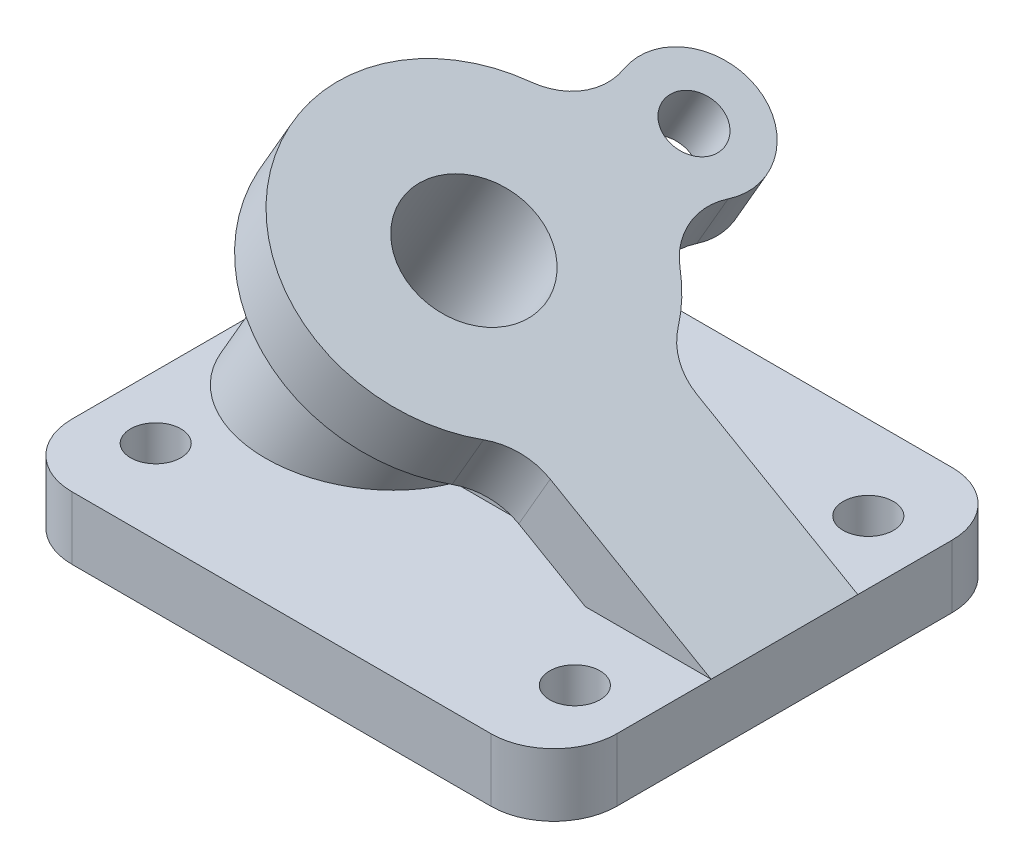
ISO-10303-21;
HEADER;
FILE_DESCRIPTION(('STEP AP214'),'2;1');
FILE_NAME('part.step','',(''),(''),'','','');
FILE_SCHEMA(('AUTOMOTIVE_DESIGN { 1 0 10303 214 1 1 1 1 }'));
ENDSEC;
DATA;
#1=APPLICATION_CONTEXT('core data for automotive mechanical design processes');
#2=APPLICATION_PROTOCOL_DEFINITION('international standard','automotive_design',2000,#1);
#3=PRODUCT_CONTEXT('',#1,'mechanical');
#4=PRODUCT('Part','Part','',(#3));
#5=PRODUCT_RELATED_PRODUCT_CATEGORY('part','',(#4));
#6=PRODUCT_DEFINITION_FORMATION('','',#4);
#7=PRODUCT_DEFINITION_CONTEXT('part definition',#1,'design');
#8=PRODUCT_DEFINITION('design','',#6,#7);
#9=PRODUCT_DEFINITION_SHAPE('','',#8);
#10=(LENGTH_UNIT() NAMED_UNIT(*) SI_UNIT(.MILLI.,.METRE.));
#11=(NAMED_UNIT(*) PLANE_ANGLE_UNIT() SI_UNIT($,.RADIAN.));
#12=(NAMED_UNIT(*) SI_UNIT($,.STERADIAN.) SOLID_ANGLE_UNIT());
#13=UNCERTAINTY_MEASURE_WITH_UNIT(LENGTH_MEASURE(1.E-05),#10,'distance_accuracy_value','');
#14=(GEOMETRIC_REPRESENTATION_CONTEXT(3) GLOBAL_UNCERTAINTY_ASSIGNED_CONTEXT((#13)) GLOBAL_UNIT_ASSIGNED_CONTEXT((#10,
#11,#12)) REPRESENTATION_CONTEXT('',''));
#15=CARTESIAN_POINT('',(0.,0.,0.));
#16=DIRECTION('',(0.,0.,1.));
#17=DIRECTION('',(1.,0.,0.));
#18=AXIS2_PLACEMENT_3D('',#15,#16,#17);
#19=CARTESIAN_POINT('',(50.,15.,40.));
#20=DIRECTION('',(0.,1.,0.));
#21=DIRECTION('',(0.,0.,1.));
#22=AXIS2_PLACEMENT_3D('',#19,#20,#21);
#23=PLANE('',#22);
#24=DIRECTION('',(1.,0.,0.));
#25=VECTOR('',#24,1.);
#26=CARTESIAN_POINT('',(50.,15.,17.5));
#27=LINE('',#26,#25);
#28=CARTESIAN_POINT('',(34.9999999999997,15.,17.5));
#29=VERTEX_POINT('',#28);
#30=CARTESIAN_POINT('',(65.,15.,17.5));
#31=VERTEX_POINT('',#30);
#32=EDGE_CURVE('E56',#29,#31,#27,.T.);
#33=ORIENTED_EDGE('',*,*,#32,.F.);
#34=DIRECTION('',(0.,0.,-1.));
#35=VECTOR('',#34,1.);
#36=CARTESIAN_POINT('',(34.9999999999997,15.,40.));
#37=LINE('',#36,#35);
#38=CARTESIAN_POINT('',(34.9999999999996,15.,7.5));
#39=VERTEX_POINT('',#38);
#40=EDGE_CURVE('E213',#29,#39,#37,.T.);
#41=ORIENTED_EDGE('',*,*,#40,.T.);
#42=DIRECTION('',(-1.,0.,0.));
#43=VECTOR('',#42,1.);
#44=CARTESIAN_POINT('',(-16.2509999999997,15.,7.5));
#45=LINE('',#44,#43);
#46=CARTESIAN_POINT('',(-6.24198056079765,15.,7.5));
#47=VERTEX_POINT('',#46);
#48=EDGE_CURVE('E304',#39,#47,#45,.T.);
#49=ORIENTED_EDGE('',*,*,#48,.T.);
#50=CARTESIAN_POINT('',(-33.7798332972281,15.,0.));
#51=DIRECTION('',(0.,1.,0.));
#52=DIRECTION('',(1.,0.,0.));
#53=AXIS2_PLACEMENT_3D('',#50,#51,#52);
#54=ELLIPSE('',#53,28.8675134594812,25.);
#55=CARTESIAN_POINT('',(-6.24198056079765,15.,-7.5));
#56=VERTEX_POINT('',#55);
#57=EDGE_CURVE('E300',#56,#47,#54,.T.);
#58=ORIENTED_EDGE('',*,*,#57,.F.);
#59=DIRECTION('',(-1.,0.,0.));
#60=VECTOR('',#59,1.);
#61=CARTESIAN_POINT('',(-16.2509999999997,15.,-7.5));
#62=LINE('',#61,#60);
#63=CARTESIAN_POINT('',(34.9999999999996,15.,-7.5));
#64=VERTEX_POINT('',#63);
#65=EDGE_CURVE('E298',#64,#56,#62,.T.);
#66=ORIENTED_EDGE('',*,*,#65,.F.);
#67=CARTESIAN_POINT('',(34.9999999999997,15.,-17.5));
#68=VERTEX_POINT('',#67);
#69=EDGE_CURVE('E68',#64,#68,#37,.T.);
#70=ORIENTED_EDGE('',*,*,#69,.T.);
#71=DIRECTION('',(1.,0.,0.));
#72=VECTOR('',#71,1.);
#73=CARTESIAN_POINT('',(50.,15.,-17.5));
#74=LINE('',#73,#72);
#75=CARTESIAN_POINT('',(65.,15.,-17.5));
#76=VERTEX_POINT('',#75);
#77=EDGE_CURVE('E284',#68,#76,#74,.T.);
#78=ORIENTED_EDGE('',*,*,#77,.T.);
#79=DIRECTION('',(0.,0.,-1.));
#80=VECTOR('',#79,1.);
#81=CARTESIAN_POINT('',(65.,15.,-39.9999999999999));
#82=LINE('',#81,#80);
#83=CARTESIAN_POINT('',(65.,15.,-39.9999999999999));
#84=VERTEX_POINT('',#83);
#85=EDGE_CURVE('E335',#76,#84,#82,.T.);
#86=ORIENTED_EDGE('',*,*,#85,.T.);
#87=CARTESIAN_POINT('',(50.,15.,-40.));
#88=DIRECTION('',(0.,1.,0.));
#89=DIRECTION('',(0.,0.,-1.));
#90=AXIS2_PLACEMENT_3D('',#87,#88,#89);
#91=CIRCLE('',#90,15.);
#92=CARTESIAN_POINT('',(49.9999999999999,15.,-55.));
#93=VERTEX_POINT('',#92);
#94=EDGE_CURVE('E338',#84,#93,#91,.T.);
#95=ORIENTED_EDGE('',*,*,#94,.T.);
#96=DIRECTION('',(-1.,0.,0.));
#97=VECTOR('',#96,1.);
#98=CARTESIAN_POINT('',(-49.9999999999999,15.,-55.));
#99=LINE('',#98,#97);
#100=CARTESIAN_POINT('',(-49.9999999999999,15.,-55.));
#101=VERTEX_POINT('',#100);
#102=EDGE_CURVE('E337',#93,#101,#99,.T.);
#103=ORIENTED_EDGE('',*,*,#102,.T.);
#104=CARTESIAN_POINT('',(-50.,15.,-40.));
#105=DIRECTION('',(0.,1.,0.));
#106=DIRECTION('',(0.,0.,1.));
#107=AXIS2_PLACEMENT_3D('',#104,#105,#106);
#108=CIRCLE('',#107,15.);
#109=CARTESIAN_POINT('',(-65.,15.,-39.9999999999999));
#110=VERTEX_POINT('',#109);
#111=EDGE_CURVE('E336',#101,#110,#108,.T.);
#112=ORIENTED_EDGE('',*,*,#111,.T.);
#113=DIRECTION('',(0.,0.,1.));
#114=VECTOR('',#113,1.);
#115=CARTESIAN_POINT('',(-65.,15.,-39.9999999999999));
#116=LINE('',#115,#114);
#117=CARTESIAN_POINT('',(-65.,15.,39.9999999999999));
#118=VERTEX_POINT('',#117);
#119=EDGE_CURVE('E344',#110,#118,#116,.T.);
#120=ORIENTED_EDGE('',*,*,#119,.T.);
#121=CARTESIAN_POINT('',(-50.,15.,40.));
#122=DIRECTION('',(0.,1.,0.));
#123=DIRECTION('',(0.,0.,1.));
#124=AXIS2_PLACEMENT_3D('',#121,#122,#123);
#125=CIRCLE('',#124,15.);
#126=CARTESIAN_POINT('',(-49.9999999999999,15.,55.));
#127=VERTEX_POINT('',#126);
#128=EDGE_CURVE('E345',#118,#127,#125,.T.);
#129=ORIENTED_EDGE('',*,*,#128,.T.);
#130=DIRECTION('',(1.,0.,0.));
#131=VECTOR('',#130,1.);
#132=CARTESIAN_POINT('',(-49.9999999999999,15.,55.));
#133=LINE('',#132,#131);
#134=CARTESIAN_POINT('',(49.9999999999999,15.,55.));
#135=VERTEX_POINT('',#134);
#136=EDGE_CURVE('E347',#127,#135,#133,.T.);
#137=ORIENTED_EDGE('',*,*,#136,.T.);
#138=CARTESIAN_POINT('',(50.,15.,40.));
#139=DIRECTION('',(0.,1.,0.));
#140=DIRECTION('',(0.,0.,1.));
#141=AXIS2_PLACEMENT_3D('',#138,#139,#140);
#142=CIRCLE('',#141,15.);
#143=CARTESIAN_POINT('',(65.,15.,39.9999999999999));
#144=VERTEX_POINT('',#143);
#145=EDGE_CURVE('E328',#135,#144,#142,.T.);
#146=ORIENTED_EDGE('',*,*,#145,.T.);
#147=EDGE_CURVE('E331',#144,#31,#82,.T.);
#148=ORIENTED_EDGE('',*,*,#147,.T.);
#149=EDGE_LOOP('',(#33,#41,#49,#58,#66,#70,#78,#86,#95,#103,#112,#120,#129,#137,#146,#148));
#150=FACE_BOUND('',#149,.T.);
#151=CARTESIAN_POINT('',(50.,15.,35.));
#152=DIRECTION('',(0.,1.,0.));
#153=DIRECTION('',(0.,0.,-1.));
#154=AXIS2_PLACEMENT_3D('',#151,#152,#153);
#155=CIRCLE('',#154,6.);
#156=CARTESIAN_POINT('',(50.,15.,29.));
#157=VERTEX_POINT('',#156);
#158=EDGE_CURVE('E313',#157,#157,#155,.T.);
#159=ORIENTED_EDGE('',*,*,#158,.F.);
#160=EDGE_LOOP('',(#159));
#161=FACE_BOUND('',#160,.T.);
#162=CARTESIAN_POINT('',(-50.,15.,-35.));
#163=DIRECTION('',(0.,1.,0.));
#164=DIRECTION('',(0.,0.,1.));
#165=AXIS2_PLACEMENT_3D('',#162,#163,#164);
#166=CIRCLE('',#165,6.);
#167=CARTESIAN_POINT('',(-50.,15.,-29.));
#168=VERTEX_POINT('',#167);
#169=EDGE_CURVE('E323',#168,#168,#166,.T.);
#170=ORIENTED_EDGE('',*,*,#169,.F.);
#171=EDGE_LOOP('',(#170));
#172=FACE_BOUND('',#171,.T.);
#173=CARTESIAN_POINT('',(-50.,15.,35.));
#174=DIRECTION('',(0.,1.,0.));
#175=DIRECTION('',(0.,0.,1.));
#176=AXIS2_PLACEMENT_3D('',#173,#174,#175);
#177=CIRCLE('',#176,6.);
#178=CARTESIAN_POINT('',(-50.,15.,41.));
#179=VERTEX_POINT('',#178);
#180=EDGE_CURVE('E320',#179,#179,#177,.T.);
#181=ORIENTED_EDGE('',*,*,#180,.F.);
#182=EDGE_LOOP('',(#181));
#183=FACE_BOUND('',#182,.T.);
#184=CARTESIAN_POINT('',(50.,15.,-35.));
#185=DIRECTION('',(0.,1.,0.));
#186=DIRECTION('',(0.,0.,-1.));
#187=AXIS2_PLACEMENT_3D('',#184,#185,#186);
#188=CIRCLE('',#187,6.);
#189=CARTESIAN_POINT('',(50.,15.,-41.));
#190=VERTEX_POINT('',#189);
#191=EDGE_CURVE('E301',#190,#190,#188,.T.);
#192=ORIENTED_EDGE('',*,*,#191,.F.);
#193=EDGE_LOOP('',(#192));
#194=FACE_BOUND('',#193,.T.);
#195=ADVANCED_FACE('F43',(#150,#161,#172,#183,#194),#23,.T.);
#196=CARTESIAN_POINT('',(50.,0.,40.));
#197=DIRECTION('',(0.,1.,0.));
#198=DIRECTION('',(0.,0.,1.));
#199=AXIS2_PLACEMENT_3D('',#196,#197,#198);
#200=PLANE('',#199);
#201=CARTESIAN_POINT('',(50.,0.,40.));
#202=DIRECTION('',(0.,1.,0.));
#203=DIRECTION('',(0.,0.,1.));
#204=AXIS2_PLACEMENT_3D('',#201,#202,#203);
#205=CIRCLE('',#204,15.);
#206=CARTESIAN_POINT('',(49.9999999999999,0.,55.));
#207=VERTEX_POINT('',#206);
#208=CARTESIAN_POINT('',(65.,0.,39.9999999999999));
#209=VERTEX_POINT('',#208);
#210=EDGE_CURVE('E326',#207,#209,#205,.T.);
#211=ORIENTED_EDGE('',*,*,#210,.F.);
#212=DIRECTION('',(1.,0.,0.));
#213=VECTOR('',#212,1.);
#214=CARTESIAN_POINT('',(-49.9999999999999,0.,55.));
#215=LINE('',#214,#213);
#216=CARTESIAN_POINT('',(-49.9999999999999,0.,55.));
#217=VERTEX_POINT('',#216);
#218=EDGE_CURVE('E334',#217,#207,#215,.T.);
#219=ORIENTED_EDGE('',*,*,#218,.F.);
#220=CARTESIAN_POINT('',(-50.,0.,40.));
#221=DIRECTION('',(0.,1.,0.));
#222=DIRECTION('',(0.,0.,1.));
#223=AXIS2_PLACEMENT_3D('',#220,#221,#222);
#224=CIRCLE('',#223,15.);
#225=CARTESIAN_POINT('',(-65.,0.,39.9999999999999));
#226=VERTEX_POINT('',#225);
#227=EDGE_CURVE('E363',#226,#217,#224,.T.);
#228=ORIENTED_EDGE('',*,*,#227,.F.);
#229=DIRECTION('',(0.,0.,1.));
#230=VECTOR('',#229,1.);
#231=CARTESIAN_POINT('',(-65.,0.,-39.9999999999999));
#232=LINE('',#231,#230);
#233=CARTESIAN_POINT('',(-65.,0.,-39.9999999999999));
#234=VERTEX_POINT('',#233);
#235=EDGE_CURVE('E360',#234,#226,#232,.T.);
#236=ORIENTED_EDGE('',*,*,#235,.F.);
#237=CARTESIAN_POINT('',(-50.,0.,-40.));
#238=DIRECTION('',(0.,1.,0.));
#239=DIRECTION('',(0.,0.,1.));
#240=AXIS2_PLACEMENT_3D('',#237,#238,#239);
#241=CIRCLE('',#240,15.);
#242=CARTESIAN_POINT('',(-49.9999999999999,0.,-55.));
#243=VERTEX_POINT('',#242);
#244=EDGE_CURVE('E359',#243,#234,#241,.T.);
#245=ORIENTED_EDGE('',*,*,#244,.F.);
#246=DIRECTION('',(-1.,0.,0.));
#247=VECTOR('',#246,1.);
#248=CARTESIAN_POINT('',(-49.9999999999999,0.,-55.));
#249=LINE('',#248,#247);
#250=CARTESIAN_POINT('',(49.9999999999999,0.,-55.));
#251=VERTEX_POINT('',#250);
#252=EDGE_CURVE('E351',#251,#243,#249,.T.);
#253=ORIENTED_EDGE('',*,*,#252,.F.);
#254=CARTESIAN_POINT('',(50.,0.,-40.));
#255=DIRECTION('',(0.,1.,0.));
#256=DIRECTION('',(0.,0.,-1.));
#257=AXIS2_PLACEMENT_3D('',#254,#255,#256);
#258=CIRCLE('',#257,15.);
#259=CARTESIAN_POINT('',(65.,0.,-39.9999999999999));
#260=VERTEX_POINT('',#259);
#261=EDGE_CURVE('E352',#260,#251,#258,.T.);
#262=ORIENTED_EDGE('',*,*,#261,.F.);
#263=DIRECTION('',(0.,0.,-1.));
#264=VECTOR('',#263,1.);
#265=CARTESIAN_POINT('',(65.,0.,-39.9999999999999));
#266=LINE('',#265,#264);
#267=EDGE_CURVE('E353',#209,#260,#266,.T.);
#268=ORIENTED_EDGE('',*,*,#267,.F.);
#269=EDGE_LOOP('',(#211,#219,#228,#236,#245,#253,#262,#268));
#270=FACE_BOUND('',#269,.T.);
#271=CARTESIAN_POINT('',(-50.,0.,-35.));
#272=DIRECTION('',(0.,1.,0.));
#273=DIRECTION('',(0.,0.,1.));
#274=AXIS2_PLACEMENT_3D('',#271,#272,#273);
#275=CIRCLE('',#274,6.);
#276=CARTESIAN_POINT('',(-50.,0.,-29.));
#277=VERTEX_POINT('',#276);
#278=EDGE_CURVE('E319',#277,#277,#275,.T.);
#279=ORIENTED_EDGE('',*,*,#278,.T.);
#280=EDGE_LOOP('',(#279));
#281=FACE_BOUND('',#280,.T.);
#282=CARTESIAN_POINT('',(-50.,0.,35.));
#283=DIRECTION('',(0.,1.,0.));
#284=DIRECTION('',(0.,0.,1.));
#285=AXIS2_PLACEMENT_3D('',#282,#283,#284);
#286=CIRCLE('',#285,6.);
#287=CARTESIAN_POINT('',(-50.,0.,41.));
#288=VERTEX_POINT('',#287);
#289=EDGE_CURVE('E314',#288,#288,#286,.T.);
#290=ORIENTED_EDGE('',*,*,#289,.T.);
#291=EDGE_LOOP('',(#290));
#292=FACE_BOUND('',#291,.T.);
#293=CARTESIAN_POINT('',(50.,0.,35.));
#294=DIRECTION('',(0.,1.,0.));
#295=DIRECTION('',(0.,0.,-1.));
#296=AXIS2_PLACEMENT_3D('',#293,#294,#295);
#297=CIRCLE('',#296,6.);
#298=CARTESIAN_POINT('',(50.,0.,29.));
#299=VERTEX_POINT('',#298);
#300=EDGE_CURVE('E306',#299,#299,#297,.T.);
#301=ORIENTED_EDGE('',*,*,#300,.T.);
#302=EDGE_LOOP('',(#301));
#303=FACE_BOUND('',#302,.T.);
#304=CARTESIAN_POINT('',(50.,0.,-35.));
#305=DIRECTION('',(0.,1.,0.));
#306=DIRECTION('',(0.,0.,-1.));
#307=AXIS2_PLACEMENT_3D('',#304,#305,#306);
#308=CIRCLE('',#307,6.);
#309=CARTESIAN_POINT('',(50.,0.,-41.));
#310=VERTEX_POINT('',#309);
#311=EDGE_CURVE('E302',#310,#310,#308,.T.);
#312=ORIENTED_EDGE('',*,*,#311,.T.);
#313=EDGE_LOOP('',(#312));
#314=FACE_BOUND('',#313,.T.);
#315=ADVANCED_FACE('F398',(#270,#281,#292,#303,#314),#200,.F.);
#316=CARTESIAN_POINT('',(50.,15.,40.));
#317=DIRECTION('',(0.,-1.,0.));
#318=DIRECTION('',(0.,0.,-1.));
#319=AXIS2_PLACEMENT_3D('',#316,#317,#318);
#320=CYLINDRICAL_SURFACE('',#319,15.);
#321=ORIENTED_EDGE('',*,*,#210,.T.);
#322=DIRECTION('',(0.,-1.,0.));
#323=VECTOR('',#322,1.);
#324=CARTESIAN_POINT('',(65.,15.,39.9999999999999));
#325=LINE('',#324,#323);
#326=EDGE_CURVE('E50',#144,#209,#325,.T.);
#327=ORIENTED_EDGE('',*,*,#326,.F.);
#328=ORIENTED_EDGE('',*,*,#145,.F.);
#329=DIRECTION('',(0.,-1.,0.));
#330=VECTOR('',#329,1.);
#331=CARTESIAN_POINT('',(49.9999999999999,15.,55.));
#332=LINE('',#331,#330);
#333=EDGE_CURVE('E346',#135,#207,#332,.T.);
#334=ORIENTED_EDGE('',*,*,#333,.T.);
#335=EDGE_LOOP('',(#321,#327,#328,#334));
#336=FACE_BOUND('',#335,.T.);
#337=ADVANCED_FACE('F44',(#336),#320,.T.);
#338=CARTESIAN_POINT('',(65.,15.,-39.9999999999999));
#339=DIRECTION('',(-1.,0.,0.));
#340=DIRECTION('',(0.,0.,1.));
#341=AXIS2_PLACEMENT_3D('',#338,#339,#340);
#342=PLANE('',#341);
#343=ORIENTED_EDGE('',*,*,#267,.T.);
#344=DIRECTION('',(0.,-1.,0.));
#345=VECTOR('',#344,1.);
#346=CARTESIAN_POINT('',(65.,15.,-39.9999999999999));
#347=LINE('',#346,#345);
#348=EDGE_CURVE('E379',#84,#260,#347,.T.);
#349=ORIENTED_EDGE('',*,*,#348,.F.);
#350=ORIENTED_EDGE('',*,*,#85,.F.);
#351=DIRECTION('',(0.,0.,-1.));
#352=VECTOR('',#351,1.);
#353=CARTESIAN_POINT('',(65.,15.,0.));
#354=LINE('',#353,#352);
#355=EDGE_CURVE('E239',#31,#76,#354,.T.);
#356=ORIENTED_EDGE('',*,*,#355,.F.);
#357=ORIENTED_EDGE('',*,*,#147,.F.);
#358=ORIENTED_EDGE('',*,*,#326,.T.);
#359=EDGE_LOOP('',(#343,#349,#350,#356,#357,#358));
#360=FACE_BOUND('',#359,.T.);
#361=ADVANCED_FACE('F386',(#360),#342,.F.);
#362=CARTESIAN_POINT('',(50.,15.,-40.));
#363=DIRECTION('',(0.,-1.,0.));
#364=DIRECTION('',(0.,0.,-1.));
#365=AXIS2_PLACEMENT_3D('',#362,#363,#364);
#366=CYLINDRICAL_SURFACE('',#365,15.);
#367=ORIENTED_EDGE('',*,*,#261,.T.);
#368=DIRECTION('',(0.,-1.,0.));
#369=VECTOR('',#368,1.);
#370=CARTESIAN_POINT('',(49.9999999999999,15.,-55.));
#371=LINE('',#370,#369);
#372=EDGE_CURVE('E378',#93,#251,#371,.T.);
#373=ORIENTED_EDGE('',*,*,#372,.F.);
#374=ORIENTED_EDGE('',*,*,#94,.F.);
#375=ORIENTED_EDGE('',*,*,#348,.T.);
#376=EDGE_LOOP('',(#367,#373,#374,#375));
#377=FACE_BOUND('',#376,.T.);
#378=ADVANCED_FACE('F405',(#377),#366,.T.);
#379=CARTESIAN_POINT('',(-49.9999999999999,15.,-55.));
#380=DIRECTION('',(0.,0.,1.));
#381=DIRECTION('',(1.,0.,0.));
#382=AXIS2_PLACEMENT_3D('',#379,#380,#381);
#383=PLANE('',#382);
#384=ORIENTED_EDGE('',*,*,#252,.T.);
#385=DIRECTION('',(0.,-1.,0.));
#386=VECTOR('',#385,1.);
#387=CARTESIAN_POINT('',(-49.9999999999999,15.,-55.));
#388=LINE('',#387,#386);
#389=EDGE_CURVE('E374',#101,#243,#388,.T.);
#390=ORIENTED_EDGE('',*,*,#389,.F.);
#391=ORIENTED_EDGE('',*,*,#102,.F.);
#392=ORIENTED_EDGE('',*,*,#372,.T.);
#393=EDGE_LOOP('',(#384,#390,#391,#392));
#394=FACE_BOUND('',#393,.T.);
#395=ADVANCED_FACE('F403',(#394),#383,.F.);
#396=CARTESIAN_POINT('',(-50.,15.,-40.));
#397=DIRECTION('',(0.,-1.,0.));
#398=DIRECTION('',(0.,0.,-1.));
#399=AXIS2_PLACEMENT_3D('',#396,#397,#398);
#400=CYLINDRICAL_SURFACE('',#399,15.);
#401=ORIENTED_EDGE('',*,*,#244,.T.);
#402=DIRECTION('',(0.,-1.,0.));
#403=VECTOR('',#402,1.);
#404=CARTESIAN_POINT('',(-65.,15.,-39.9999999999999));
#405=LINE('',#404,#403);
#406=EDGE_CURVE('E375',#110,#234,#405,.T.);
#407=ORIENTED_EDGE('',*,*,#406,.F.);
#408=ORIENTED_EDGE('',*,*,#111,.F.);
#409=ORIENTED_EDGE('',*,*,#389,.T.);
#410=EDGE_LOOP('',(#401,#407,#408,#409));
#411=FACE_BOUND('',#410,.T.);
#412=ADVANCED_FACE('F666',(#411),#400,.T.);
#413=CARTESIAN_POINT('',(-65.,15.,-39.9999999999999));
#414=DIRECTION('',(1.,0.,0.));
#415=DIRECTION('',(0.,0.,-1.));
#416=AXIS2_PLACEMENT_3D('',#413,#414,#415);
#417=PLANE('',#416);
#418=ORIENTED_EDGE('',*,*,#235,.T.);
#419=DIRECTION('',(0.,-1.,0.));
#420=VECTOR('',#419,1.);
#421=CARTESIAN_POINT('',(-65.,15.,39.9999999999999));
#422=LINE('',#421,#420);
#423=EDGE_CURVE('E369',#118,#226,#422,.T.);
#424=ORIENTED_EDGE('',*,*,#423,.F.);
#425=ORIENTED_EDGE('',*,*,#119,.F.);
#426=ORIENTED_EDGE('',*,*,#406,.T.);
#427=EDGE_LOOP('',(#418,#424,#425,#426));
#428=FACE_BOUND('',#427,.T.);
#429=ADVANCED_FACE('F659',(#428),#417,.F.);
#430=CARTESIAN_POINT('',(-50.,15.,40.));
#431=DIRECTION('',(0.,-1.,0.));
#432=DIRECTION('',(0.,0.,-1.));
#433=AXIS2_PLACEMENT_3D('',#430,#431,#432);
#434=CYLINDRICAL_SURFACE('',#433,15.);
#435=ORIENTED_EDGE('',*,*,#227,.T.);
#436=DIRECTION('',(0.,-1.,0.));
#437=VECTOR('',#436,1.);
#438=CARTESIAN_POINT('',(-49.9999999999999,15.,55.));
#439=LINE('',#438,#437);
#440=EDGE_CURVE('E368',#127,#217,#439,.T.);
#441=ORIENTED_EDGE('',*,*,#440,.F.);
#442=ORIENTED_EDGE('',*,*,#128,.F.);
#443=ORIENTED_EDGE('',*,*,#423,.T.);
#444=EDGE_LOOP('',(#435,#441,#442,#443));
#445=FACE_BOUND('',#444,.T.);
#446=ADVANCED_FACE('F649',(#445),#434,.T.);
#447=CARTESIAN_POINT('',(-49.9999999999999,15.,55.));
#448=DIRECTION('',(0.,0.,-1.));
#449=DIRECTION('',(-1.,0.,0.));
#450=AXIS2_PLACEMENT_3D('',#447,#448,#449);
#451=PLANE('',#450);
#452=ORIENTED_EDGE('',*,*,#218,.T.);
#453=ORIENTED_EDGE('',*,*,#333,.F.);
#454=ORIENTED_EDGE('',*,*,#136,.F.);
#455=ORIENTED_EDGE('',*,*,#440,.T.);
#456=EDGE_LOOP('',(#452,#453,#454,#455));
#457=FACE_BOUND('',#456,.T.);
#458=ADVANCED_FACE('F643',(#457),#451,.F.);
#459=CARTESIAN_POINT('',(-50.,15.,-35.));
#460=DIRECTION('',(0.,-1.,0.));
#461=DIRECTION('',(0.,0.,-1.));
#462=AXIS2_PLACEMENT_3D('',#459,#460,#461);
#463=CYLINDRICAL_SURFACE('',#462,6.);
#464=ORIENTED_EDGE('',*,*,#169,.T.);
#465=EDGE_LOOP('',(#464));
#466=FACE_BOUND('',#465,.T.);
#467=ORIENTED_EDGE('',*,*,#278,.F.);
#468=EDGE_LOOP('',(#467));
#469=FACE_BOUND('',#468,.T.);
#470=ADVANCED_FACE('F633',(#466,#469),#463,.F.);
#471=CARTESIAN_POINT('',(-50.,15.,35.));
#472=DIRECTION('',(0.,-1.,0.));
#473=DIRECTION('',(0.,0.,-1.));
#474=AXIS2_PLACEMENT_3D('',#471,#472,#473);
#475=CYLINDRICAL_SURFACE('',#474,6.);
#476=ORIENTED_EDGE('',*,*,#180,.T.);
#477=EDGE_LOOP('',(#476));
#478=FACE_BOUND('',#477,.T.);
#479=ORIENTED_EDGE('',*,*,#289,.F.);
#480=EDGE_LOOP('',(#479));
#481=FACE_BOUND('',#480,.T.);
#482=ADVANCED_FACE('F622',(#478,#481),#475,.F.);
#483=CARTESIAN_POINT('',(50.,15.,35.));
#484=DIRECTION('',(0.,-1.,0.));
#485=DIRECTION('',(0.,0.,-1.));
#486=AXIS2_PLACEMENT_3D('',#483,#484,#485);
#487=CYLINDRICAL_SURFACE('',#486,6.);
#488=ORIENTED_EDGE('',*,*,#158,.T.);
#489=EDGE_LOOP('',(#488));
#490=FACE_BOUND('',#489,.T.);
#491=ORIENTED_EDGE('',*,*,#300,.F.);
#492=EDGE_LOOP('',(#491));
#493=FACE_BOUND('',#492,.T.);
#494=ADVANCED_FACE('F461',(#490,#493),#487,.F.);
#495=CARTESIAN_POINT('',(50.,15.,-35.));
#496=DIRECTION('',(0.,-1.,0.));
#497=DIRECTION('',(0.,0.,-1.));
#498=AXIS2_PLACEMENT_3D('',#495,#496,#497);
#499=CYLINDRICAL_SURFACE('',#498,6.);
#500=ORIENTED_EDGE('',*,*,#191,.T.);
#501=EDGE_LOOP('',(#500));
#502=FACE_BOUND('',#501,.T.);
#503=ORIENTED_EDGE('',*,*,#311,.F.);
#504=EDGE_LOOP('',(#503));
#505=FACE_BOUND('',#504,.T.);
#506=ADVANCED_FACE('F451',(#502,#505),#499,.F.);
#507=CARTESIAN_POINT('',(-48.0810655013041,-9.77046078830035,0.));
#508=DIRECTION('',(0.499999999999995,0.866025403784442,0.));
#509=DIRECTION('',(-0.866025403784442,0.499999999999995,0.));
#510=AXIS2_PLACEMENT_3D('',#507,#508,#509);
#511=CYLINDRICAL_SURFACE('',#510,25.);
#512=DIRECTION('',(0.499999999999995,0.866025403784442,0.));
#513=VECTOR('',#512,1.);
#514=CARTESIAN_POINT('',(-27.4276759489812,-21.694700806012,-7.50000000000001));
#515=LINE('',#514,#513);
#516=CARTESIAN_POINT('',(4.06851457940145,32.8583014340171,-7.5));
#517=VERTEX_POINT('',#516);
#518=EDGE_CURVE('E295',#56,#517,#515,.T.);
#519=ORIENTED_EDGE('',*,*,#518,.F.);
#520=ORIENTED_EDGE('',*,*,#57,.T.);
#521=DIRECTION('',(0.499999999999995,0.866025403784442,0.));
#522=VECTOR('',#521,1.);
#523=CARTESIAN_POINT('',(-27.4276759489812,-21.694700806012,7.49999999999999));
#524=LINE('',#523,#522);
#525=CARTESIAN_POINT('',(4.06851457940146,32.8583014340171,7.5));
#526=VERTEX_POINT('',#525);
#527=EDGE_CURVE('E294',#47,#526,#524,.T.);
#528=ORIENTED_EDGE('',*,*,#527,.T.);
#529=CARTESIAN_POINT('',(-16.5848749729215,44.7825414517288,0.));
#530=DIRECTION('',(-0.499999999999995,-0.866025403784442,0.));
#531=DIRECTION('',(0.866025403784442,-0.499999999999995,0.));
#532=AXIS2_PLACEMENT_3D('',#529,#530,#531);
#533=CIRCLE('',#532,25.);
#534=EDGE_CURVE('E288',#526,#517,#533,.T.);
#535=ORIENTED_EDGE('',*,*,#534,.T.);
#536=EDGE_LOOP('',(#519,#520,#528,#535));
#537=FACE_BOUND('',#536,.T.);
#538=ADVANCED_FACE('F447',(#537),#511,.T.);
#539=CARTESIAN_POINT('',(-16.2509999999997,-28.1475576738016,-7.50000000000001));
#540=DIRECTION('',(0.,0.,1.));
#541=DIRECTION('',(0.,-1.,0.));
#542=AXIS2_PLACEMENT_3D('',#539,#540,#541);
#543=PLANE('',#542);
#544=DIRECTION('',(0.866025403784442,-0.499999999999995,0.));
#545=VECTOR('',#544,1.);
#546=CARTESIAN_POINT('',(15.245190528383,26.4054445662275,-7.5));
#547=LINE('',#546,#545);
#548=EDGE_CURVE('E290',#517,#64,#547,.T.);
#549=ORIENTED_EDGE('',*,*,#548,.T.);
#550=ORIENTED_EDGE('',*,*,#65,.T.);
#551=ORIENTED_EDGE('',*,*,#518,.T.);
#552=EDGE_LOOP('',(#549,#550,#551));
#553=FACE_BOUND('',#552,.T.);
#554=ADVANCED_FACE('F443',(#553),#543,.F.);
#555=CARTESIAN_POINT('',(-16.2509999999997,-28.1475576738016,7.49999999999999));
#556=DIRECTION('',(0.,0.,1.));
#557=DIRECTION('',(0.,-1.,0.));
#558=AXIS2_PLACEMENT_3D('',#555,#556,#557);
#559=PLANE('',#558);
#560=ORIENTED_EDGE('',*,*,#48,.F.);
#561=DIRECTION('',(0.866025403784442,-0.499999999999995,0.));
#562=VECTOR('',#561,1.);
#563=CARTESIAN_POINT('',(15.245190528383,26.4054445662275,7.5));
#564=LINE('',#563,#562);
#565=EDGE_CURVE('E285',#526,#39,#564,.T.);
#566=ORIENTED_EDGE('',*,*,#565,.F.);
#567=ORIENTED_EDGE('',*,*,#527,.F.);
#568=EDGE_LOOP('',(#560,#566,#567));
#569=FACE_BOUND('',#568,.T.);
#570=ADVANCED_FACE('F454',(#569),#559,.T.);
#571=CARTESIAN_POINT('',(15.245190528383,26.4054445662275,0.));
#572=DIRECTION('',(0.499999999999995,0.866025403784442,0.));
#573=DIRECTION('',(-0.866025403784442,0.499999999999995,0.));
#574=AXIS2_PLACEMENT_3D('',#571,#572,#573);
#575=PLANE('',#574);
#576=ORIENTED_EDGE('',*,*,#69,.F.);
#577=ORIENTED_EDGE('',*,*,#548,.F.);
#578=ORIENTED_EDGE('',*,*,#534,.F.);
#579=ORIENTED_EDGE('',*,*,#565,.T.);
#580=ORIENTED_EDGE('',*,*,#40,.F.);
#581=DIRECTION('',(0.866025403784442,-0.499999999999995,0.));
#582=VECTOR('',#581,1.);
#583=CARTESIAN_POINT('',(15.245190528383,26.4054445662275,17.5));
#584=LINE('',#583,#582);
#585=CARTESIAN_POINT('',(19.1222671697929,24.1670133236407,17.5));
#586=VERTEX_POINT('',#585);
#587=EDGE_CURVE('E194',#586,#29,#584,.T.);
#588=ORIENTED_EDGE('',*,*,#587,.F.);
#589=CARTESIAN_POINT('',(19.1222671697929,24.1670133236407,32.5));
#590=DIRECTION('',(0.499999999999995,0.866025403784442,0.));
#591=DIRECTION('',(-0.866025403784442,0.499999999999995,0.));
#592=AXIS2_PLACEMENT_3D('',#589,#590,#591);
#593=CIRCLE('',#592,15.);
#594=CARTESIAN_POINT('',(8.92022655758879,30.0571642173801,23.2142857142857));
#595=VERTEX_POINT('',#594);
#596=EDGE_CURVE('E205',#586,#595,#593,.T.);
#597=ORIENTED_EDGE('',*,*,#596,.T.);
#598=CARTESIAN_POINT('',(-16.5848749729215,44.7825414517288,0.));
#599=DIRECTION('',(0.499999999999995,0.866025403784442,0.));
#600=DIRECTION('',(-0.866025403784442,0.499999999999995,0.));
#601=AXIS2_PLACEMENT_3D('',#598,#599,#600);
#602=CIRCLE('',#601,37.5);
#603=CARTESIAN_POINT('',(-34.3689821748944,55.0502005320849,-31.3775510204082));
#604=VERTEX_POINT('',#603);
#605=EDGE_CURVE('E234',#604,#595,#602,.T.);
#606=ORIENTED_EDGE('',*,*,#605,.F.);
#607=CARTESIAN_POINT('',(-41.4826250556835,59.1572641642273,-43.9285714285714));
#608=DIRECTION('',(0.499999999999995,0.866025403784442,0.));
#609=DIRECTION('',(-0.866025403784442,0.499999999999995,0.));
#610=AXIS2_PLACEMENT_3D('',#607,#608,#609);
#611=CIRCLE('',#610,15.);
#612=CARTESIAN_POINT('',(-29.0337500143025,51.969902807978,-48.2142857142857));
#613=VERTEX_POINT('',#612);
#614=EDGE_CURVE('E226',#604,#613,#611,.T.);
#615=ORIENTED_EDGE('',*,*,#614,.T.);
#616=CARTESIAN_POINT('',(-16.5848749729215,44.7825414517288,-52.5));
#617=DIRECTION('',(0.499999999999995,0.866025403784442,0.));
#618=DIRECTION('',(-0.866025403784442,0.499999999999995,0.));
#619=AXIS2_PLACEMENT_3D('',#616,#617,#618);
#620=CIRCLE('',#619,15.);
#621=CARTESIAN_POINT('',(-4.13599993154047,37.5951800954795,-48.2142857142857));
#622=VERTEX_POINT('',#621);
#623=EDGE_CURVE('E229',#622,#613,#620,.T.);
#624=ORIENTED_EDGE('',*,*,#623,.F.);
#625=CARTESIAN_POINT('',(8.31287510984055,30.4078187392303,-43.9285714285714));
#626=DIRECTION('',(0.499999999999995,0.866025403784442,0.));
#627=DIRECTION('',(-0.866025403784442,0.499999999999995,0.));
#628=AXIS2_PLACEMENT_3D('',#625,#626,#627);
#629=CIRCLE('',#628,15.);
#630=CARTESIAN_POINT('',(1.1992322290514,34.5148823713727,-31.3775510204082));
#631=VERTEX_POINT('',#630);
#632=EDGE_CURVE('E223',#622,#631,#629,.T.);
#633=ORIENTED_EDGE('',*,*,#632,.T.);
#634=CARTESIAN_POINT('',(-16.5848749729215,44.7825414517288,0.));
#635=DIRECTION('',(0.499999999999995,0.866025403784442,0.));
#636=DIRECTION('',(-0.866025403784442,0.499999999999995,0.));
#637=AXIS2_PLACEMENT_3D('',#634,#635,#636);
#638=CIRCLE('',#637,37.5);
#639=CARTESIAN_POINT('',(8.92022655758878,30.0571642173801,-23.2142857142857));
#640=VERTEX_POINT('',#639);
#641=EDGE_CURVE('E225',#640,#631,#638,.T.);
#642=ORIENTED_EDGE('',*,*,#641,.F.);
#643=CARTESIAN_POINT('',(19.1222671697929,24.1670133236407,-32.5));
#644=DIRECTION('',(0.499999999999995,0.866025403784442,0.));
#645=DIRECTION('',(-0.866025403784442,0.499999999999995,0.));
#646=AXIS2_PLACEMENT_3D('',#643,#644,#645);
#647=CIRCLE('',#646,15.);
#648=CARTESIAN_POINT('',(19.1222671697929,24.1670133236407,-17.5));
#649=VERTEX_POINT('',#648);
#650=EDGE_CURVE('E220',#649,#640,#647,.F.);
#651=ORIENTED_EDGE('',*,*,#650,.F.);
#652=DIRECTION('',(0.866025403784442,-0.499999999999995,0.));
#653=VECTOR('',#652,1.);
#654=CARTESIAN_POINT('',(15.245190528383,26.4054445662275,-17.5));
#655=LINE('',#654,#653);
#656=EDGE_CURVE('E212',#649,#68,#655,.T.);
#657=ORIENTED_EDGE('',*,*,#656,.T.);
#658=EDGE_LOOP('',(#576,#577,#578,#579,#580,#588,#597,#606,#615,#624,#633,#642,#651,#657));
#659=FACE_BOUND('',#658,.T.);
#660=CARTESIAN_POINT('',(-16.5848749729215,44.7825414517288,-52.5));
#661=DIRECTION('',(0.499999999999995,0.866025403784442,0.));
#662=DIRECTION('',(-0.866025403784442,0.499999999999995,0.));
#663=AXIS2_PLACEMENT_3D('',#660,#661,#662);
#664=CIRCLE('',#663,6.50000000000001);
#665=CARTESIAN_POINT('',(-22.2140400975204,48.0325414517288,-52.5));
#666=VERTEX_POINT('',#665);
#667=EDGE_CURVE('E200',#666,#666,#664,.T.);
#668=ORIENTED_EDGE('',*,*,#667,.T.);
#669=EDGE_LOOP('',(#668));
#670=FACE_BOUND('',#669,.T.);
#671=ADVANCED_FACE('F209',(#659,#670),#575,.F.);
#672=CARTESIAN_POINT('',(19.1222671697929,24.1670133236407,32.5));
#673=DIRECTION('',(0.499999999999995,0.866025403784442,0.));
#674=DIRECTION('',(-0.866025403784442,0.499999999999995,0.));
#675=AXIS2_PLACEMENT_3D('',#672,#673,#674);
#676=CYLINDRICAL_SURFACE('',#675,15.);
#677=CARTESIAN_POINT('',(26.6222671697928,37.1573943804073,32.5));
#678=DIRECTION('',(0.499999999999995,0.866025403784442,0.));
#679=DIRECTION('',(-0.866025403784442,0.499999999999995,0.));
#680=AXIS2_PLACEMENT_3D('',#677,#678,#679);
#681=CIRCLE('',#680,15.);
#682=CARTESIAN_POINT('',(26.6222671697928,37.1573943804073,17.5));
#683=VERTEX_POINT('',#682);
#684=CARTESIAN_POINT('',(16.4202265575887,43.0475452741468,23.2142857142857));
#685=VERTEX_POINT('',#684);
#686=EDGE_CURVE('E237',#683,#685,#681,.T.);
#687=ORIENTED_EDGE('',*,*,#686,.T.);
#688=DIRECTION('',(0.499999999999995,0.866025403784442,0.));
#689=VECTOR('',#688,1.);
#690=CARTESIAN_POINT('',(8.92022655758879,30.0571642173801,23.2142857142857));
#691=LINE('',#690,#689);
#692=EDGE_CURVE('E204',#595,#685,#691,.T.);
#693=ORIENTED_EDGE('',*,*,#692,.F.);
#694=ORIENTED_EDGE('',*,*,#596,.F.);
#695=DIRECTION('',(0.499999999999995,0.866025403784442,0.));
#696=VECTOR('',#695,1.);
#697=CARTESIAN_POINT('',(19.1222671697929,24.1670133236407,17.5));
#698=LINE('',#697,#696);
#699=EDGE_CURVE('E187',#586,#683,#698,.T.);
#700=ORIENTED_EDGE('',*,*,#699,.T.);
#701=EDGE_LOOP('',(#687,#693,#694,#700));
#702=FACE_BOUND('',#701,.T.);
#703=ADVANCED_FACE('F201',(#702),#676,.F.);
#704=CARTESIAN_POINT('',(-16.5848749729215,44.7825414517288,0.));
#705=DIRECTION('',(0.499999999999995,0.866025403784442,0.));
#706=DIRECTION('',(-0.866025403784442,0.499999999999995,0.));
#707=AXIS2_PLACEMENT_3D('',#704,#705,#706);
#708=CYLINDRICAL_SURFACE('',#707,37.5);
#709=CARTESIAN_POINT('',(-9.08487497292158,57.7729225084954,0.));
#710=DIRECTION('',(0.499999999999995,0.866025403784442,0.));
#711=DIRECTION('',(-0.866025403784442,0.499999999999995,0.));
#712=AXIS2_PLACEMENT_3D('',#709,#710,#711);
#713=CIRCLE('',#712,37.5);
#714=CARTESIAN_POINT('',(-26.8689821748945,68.0405815888515,-31.3775510204082));
#715=VERTEX_POINT('',#714);
#716=EDGE_CURVE('E257',#715,#685,#713,.T.);
#717=ORIENTED_EDGE('',*,*,#716,.F.);
#718=DIRECTION('',(0.499999999999995,0.866025403784442,0.));
#719=VECTOR('',#718,1.);
#720=CARTESIAN_POINT('',(-34.3689821748944,55.0502005320849,-31.3775510204082));
#721=LINE('',#720,#719);
#722=EDGE_CURVE('E267',#604,#715,#721,.T.);
#723=ORIENTED_EDGE('',*,*,#722,.F.);
#724=ORIENTED_EDGE('',*,*,#605,.T.);
#725=ORIENTED_EDGE('',*,*,#692,.T.);
#726=EDGE_LOOP('',(#717,#723,#724,#725));
#727=FACE_BOUND('',#726,.T.);
#728=ADVANCED_FACE('F425',(#727),#708,.T.);
#729=CARTESIAN_POINT('',(-41.4826250556835,59.1572641642273,-43.9285714285714));
#730=DIRECTION('',(0.499999999999995,0.866025403784442,0.));
#731=DIRECTION('',(-0.866025403784442,0.499999999999995,0.));
#732=AXIS2_PLACEMENT_3D('',#729,#730,#731);
#733=CYLINDRICAL_SURFACE('',#732,15.);
#734=CARTESIAN_POINT('',(-33.9826250556836,72.1476452209939,-43.9285714285714));
#735=DIRECTION('',(0.499999999999995,0.866025403784442,0.));
#736=DIRECTION('',(-0.866025403784442,0.499999999999995,0.));
#737=AXIS2_PLACEMENT_3D('',#734,#735,#736);
#738=CIRCLE('',#737,15.);
#739=CARTESIAN_POINT('',(-21.5337500143026,64.9602838647446,-48.2142857142857));
#740=VERTEX_POINT('',#739);
#741=EDGE_CURVE('E260',#715,#740,#738,.T.);
#742=ORIENTED_EDGE('',*,*,#741,.T.);
#743=DIRECTION('',(0.499999999999995,0.866025403784442,0.));
#744=VECTOR('',#743,1.);
#745=CARTESIAN_POINT('',(-29.0337500143025,51.969902807978,-48.2142857142857));
#746=LINE('',#745,#744);
#747=EDGE_CURVE('E271',#613,#740,#746,.T.);
#748=ORIENTED_EDGE('',*,*,#747,.F.);
#749=ORIENTED_EDGE('',*,*,#614,.F.);
#750=ORIENTED_EDGE('',*,*,#722,.T.);
#751=EDGE_LOOP('',(#742,#748,#749,#750));
#752=FACE_BOUND('',#751,.T.);
#753=ADVANCED_FACE('F430',(#752),#733,.F.);
#754=CARTESIAN_POINT('',(-16.5848749729215,44.7825414517288,-52.5));
#755=DIRECTION('',(0.499999999999995,0.866025403784442,0.));
#756=DIRECTION('',(-0.866025403784442,0.499999999999995,0.));
#757=AXIS2_PLACEMENT_3D('',#754,#755,#756);
#758=CYLINDRICAL_SURFACE('',#757,15.);
#759=CARTESIAN_POINT('',(-9.08487497292158,57.7729225084954,-52.5));
#760=DIRECTION('',(0.499999999999995,0.866025403784442,0.));
#761=DIRECTION('',(-0.866025403784442,0.499999999999995,0.));
#762=AXIS2_PLACEMENT_3D('',#759,#760,#761);
#763=CIRCLE('',#762,15.);
#764=CARTESIAN_POINT('',(3.36400006845945,50.5855611522462,-48.2142857142857));
#765=VERTEX_POINT('',#764);
#766=EDGE_CURVE('E255',#765,#740,#763,.T.);
#767=ORIENTED_EDGE('',*,*,#766,.F.);
#768=DIRECTION('',(0.499999999999995,0.866025403784442,0.));
#769=VECTOR('',#768,1.);
#770=CARTESIAN_POINT('',(-4.13599993154047,37.5951800954795,-48.2142857142857));
#771=LINE('',#770,#769);
#772=EDGE_CURVE('E272',#622,#765,#771,.T.);
#773=ORIENTED_EDGE('',*,*,#772,.F.);
#774=ORIENTED_EDGE('',*,*,#623,.T.);
#775=ORIENTED_EDGE('',*,*,#747,.T.);
#776=EDGE_LOOP('',(#767,#773,#774,#775));
#777=FACE_BOUND('',#776,.T.);
#778=ADVANCED_FACE('F429',(#777),#758,.T.);
#779=CARTESIAN_POINT('',(8.31287510984055,30.4078187392303,-43.9285714285714));
#780=DIRECTION('',(0.499999999999995,0.866025403784442,0.));
#781=DIRECTION('',(-0.866025403784442,0.499999999999995,0.));
#782=AXIS2_PLACEMENT_3D('',#779,#780,#781);
#783=CYLINDRICAL_SURFACE('',#782,15.);
#784=CARTESIAN_POINT('',(15.8128751098405,43.3981997959969,-43.9285714285714));
#785=DIRECTION('',(0.499999999999995,0.866025403784442,0.));
#786=DIRECTION('',(-0.866025403784442,0.499999999999995,0.));
#787=AXIS2_PLACEMENT_3D('',#784,#785,#786);
#788=CIRCLE('',#787,15.);
#789=CARTESIAN_POINT('',(8.69923222905132,47.5052634281394,-31.3775510204082));
#790=VERTEX_POINT('',#789);
#791=EDGE_CURVE('E253',#765,#790,#788,.T.);
#792=ORIENTED_EDGE('',*,*,#791,.T.);
#793=DIRECTION('',(0.499999999999995,0.866025403784442,0.));
#794=VECTOR('',#793,1.);
#795=CARTESIAN_POINT('',(1.1992322290514,34.5148823713727,-31.3775510204082));
#796=LINE('',#795,#794);
#797=EDGE_CURVE('E274',#631,#790,#796,.T.);
#798=ORIENTED_EDGE('',*,*,#797,.F.);
#799=ORIENTED_EDGE('',*,*,#632,.F.);
#800=ORIENTED_EDGE('',*,*,#772,.T.);
#801=EDGE_LOOP('',(#792,#798,#799,#800));
#802=FACE_BOUND('',#801,.T.);
#803=ADVANCED_FACE('F434',(#802),#783,.F.);
#804=CARTESIAN_POINT('',(-16.5848749729215,44.7825414517288,0.));
#805=DIRECTION('',(0.499999999999995,0.866025403784442,0.));
#806=DIRECTION('',(-0.866025403784442,0.499999999999995,0.));
#807=AXIS2_PLACEMENT_3D('',#804,#805,#806);
#808=CYLINDRICAL_SURFACE('',#807,37.5);
#809=CARTESIAN_POINT('',(-9.08487497292158,57.7729225084954,0.));
#810=DIRECTION('',(0.499999999999995,0.866025403784442,0.));
#811=DIRECTION('',(-0.866025403784442,0.499999999999995,0.));
#812=AXIS2_PLACEMENT_3D('',#809,#810,#811);
#813=CIRCLE('',#812,37.5);
#814=CARTESIAN_POINT('',(16.4202265575887,43.0475452741468,-23.2142857142857));
#815=VERTEX_POINT('',#814);
#816=EDGE_CURVE('E247',#815,#790,#813,.T.);
#817=ORIENTED_EDGE('',*,*,#816,.F.);
#818=DIRECTION('',(0.499999999999995,0.866025403784442,0.));
#819=VECTOR('',#818,1.);
#820=CARTESIAN_POINT('',(8.92022655758878,30.0571642173801,-23.2142857142857));
#821=LINE('',#820,#819);
#822=EDGE_CURVE('E280',#640,#815,#821,.T.);
#823=ORIENTED_EDGE('',*,*,#822,.F.);
#824=ORIENTED_EDGE('',*,*,#641,.T.);
#825=ORIENTED_EDGE('',*,*,#797,.T.);
#826=EDGE_LOOP('',(#817,#823,#824,#825));
#827=FACE_BOUND('',#826,.T.);
#828=ADVANCED_FACE('F509',(#827),#808,.T.);
#829=CARTESIAN_POINT('',(19.1222671697929,24.1670133236407,-32.5));
#830=DIRECTION('',(0.499999999999995,0.866025403784442,0.));
#831=DIRECTION('',(-0.866025403784442,0.499999999999995,0.));
#832=AXIS2_PLACEMENT_3D('',#829,#830,#831);
#833=CYLINDRICAL_SURFACE('',#832,15.);
#834=CARTESIAN_POINT('',(26.6222671697928,37.1573943804073,-32.5));
#835=DIRECTION('',(0.499999999999995,0.866025403784442,0.));
#836=DIRECTION('',(-0.866025403784442,0.499999999999995,0.));
#837=AXIS2_PLACEMENT_3D('',#834,#835,#836);
#838=CIRCLE('',#837,15.);
#839=CARTESIAN_POINT('',(26.6222671697928,37.1573943804073,-17.5));
#840=VERTEX_POINT('',#839);
#841=EDGE_CURVE('E241',#840,#815,#838,.F.);
#842=ORIENTED_EDGE('',*,*,#841,.F.);
#843=DIRECTION('',(0.499999999999995,0.866025403784442,0.));
#844=VECTOR('',#843,1.);
#845=CARTESIAN_POINT('',(19.1222671697929,24.1670133236407,-17.5));
#846=LINE('',#845,#844);
#847=EDGE_CURVE('E196',#649,#840,#846,.T.);
#848=ORIENTED_EDGE('',*,*,#847,.F.);
#849=ORIENTED_EDGE('',*,*,#650,.T.);
#850=ORIENTED_EDGE('',*,*,#822,.T.);
#851=EDGE_LOOP('',(#842,#848,#849,#850));
#852=FACE_BOUND('',#851,.T.);
#853=ADVANCED_FACE('F439',(#852),#833,.F.);
#854=CARTESIAN_POINT('',(15.245190528383,26.4054445662275,-17.5));
#855=DIRECTION('',(0.,0.,1.));
#856=DIRECTION('',(1.,0.,0.));
#857=AXIS2_PLACEMENT_3D('',#854,#855,#856);
#858=PLANE('',#857);
#859=ORIENTED_EDGE('',*,*,#77,.F.);
#860=ORIENTED_EDGE('',*,*,#656,.F.);
#861=ORIENTED_EDGE('',*,*,#847,.T.);
#862=DIRECTION('',(0.866025403784442,-0.499999999999995,0.));
#863=VECTOR('',#862,1.);
#864=CARTESIAN_POINT('',(22.7451905283829,39.3958256229941,-17.5));
#865=LINE('',#864,#863);
#866=EDGE_CURVE('E244',#840,#76,#865,.T.);
#867=ORIENTED_EDGE('',*,*,#866,.T.);
#868=EDGE_LOOP('',(#859,#860,#861,#867));
#869=FACE_BOUND('',#868,.T.);
#870=ADVANCED_FACE('F412',(#869),#858,.F.);
#871=CARTESIAN_POINT('',(-16.5848749729215,44.7825414517288,-52.5));
#872=DIRECTION('',(0.499999999999995,0.866025403784442,0.));
#873=DIRECTION('',(-0.866025403784442,0.499999999999995,0.));
#874=AXIS2_PLACEMENT_3D('',#871,#872,#873);
#875=CYLINDRICAL_SURFACE('',#874,6.50000000000001);
#876=ORIENTED_EDGE('',*,*,#667,.F.);
#877=EDGE_LOOP('',(#876));
#878=FACE_BOUND('',#877,.T.);
#879=CARTESIAN_POINT('',(-9.08487497292158,57.7729225084954,-52.5));
#880=DIRECTION('',(0.499999999999995,0.866025403784442,0.));
#881=DIRECTION('',(-0.866025403784442,0.499999999999995,0.));
#882=AXIS2_PLACEMENT_3D('',#879,#880,#881);
#883=CIRCLE('',#882,6.50000000000001);
#884=CARTESIAN_POINT('',(-14.7140400975205,61.0229225084954,-52.5));
#885=VERTEX_POINT('',#884);
#886=EDGE_CURVE('E263',#885,#885,#883,.T.);
#887=ORIENTED_EDGE('',*,*,#886,.T.);
#888=EDGE_LOOP('',(#887));
#889=FACE_BOUND('',#888,.T.);
#890=ADVANCED_FACE('F492',(#878,#889),#875,.F.);
#891=CARTESIAN_POINT('',(15.245190528383,26.4054445662275,17.5));
#892=DIRECTION('',(0.,0.,1.));
#893=DIRECTION('',(1.,0.,0.));
#894=AXIS2_PLACEMENT_3D('',#891,#892,#893);
#895=PLANE('',#894);
#896=ORIENTED_EDGE('',*,*,#587,.T.);
#897=ORIENTED_EDGE('',*,*,#32,.T.);
#898=DIRECTION('',(0.866025403784442,-0.499999999999995,0.));
#899=VECTOR('',#898,1.);
#900=CARTESIAN_POINT('',(22.7451905283829,39.3958256229941,17.5));
#901=LINE('',#900,#899);
#902=EDGE_CURVE('E195',#683,#31,#901,.T.);
#903=ORIENTED_EDGE('',*,*,#902,.F.);
#904=ORIENTED_EDGE('',*,*,#699,.F.);
#905=EDGE_LOOP('',(#896,#897,#903,#904));
#906=FACE_BOUND('',#905,.T.);
#907=ADVANCED_FACE('F186',(#906),#895,.T.);
#908=CARTESIAN_POINT('',(22.7451905283829,39.3958256229941,0.));
#909=DIRECTION('',(0.499999999999995,0.866025403784442,0.));
#910=DIRECTION('',(-0.866025403784442,0.499999999999995,0.));
#911=AXIS2_PLACEMENT_3D('',#908,#909,#910);
#912=PLANE('',#911);
#913=ORIENTED_EDGE('',*,*,#686,.F.);
#914=ORIENTED_EDGE('',*,*,#902,.T.);
#915=ORIENTED_EDGE('',*,*,#355,.T.);
#916=ORIENTED_EDGE('',*,*,#866,.F.);
#917=ORIENTED_EDGE('',*,*,#841,.T.);
#918=ORIENTED_EDGE('',*,*,#816,.T.);
#919=ORIENTED_EDGE('',*,*,#791,.F.);
#920=ORIENTED_EDGE('',*,*,#766,.T.);
#921=ORIENTED_EDGE('',*,*,#741,.F.);
#922=ORIENTED_EDGE('',*,*,#716,.T.);
#923=EDGE_LOOP('',(#913,#914,#915,#916,#917,#918,#919,#920,#921,#922));
#924=FACE_BOUND('',#923,.T.);
#925=ORIENTED_EDGE('',*,*,#886,.F.);
#926=EDGE_LOOP('',(#925));
#927=FACE_BOUND('',#926,.T.);
#928=CARTESIAN_POINT('',(-9.08487497292157,57.7729225084954,0.));
#929=DIRECTION('',(0.499999999999995,0.866025403784442,0.));
#930=DIRECTION('',(-0.866025403784442,0.499999999999995,0.));
#931=AXIS2_PLACEMENT_3D('',#928,#929,#930);
#932=CIRCLE('',#931,15.);
#933=CARTESIAN_POINT('',(-22.0752560296882,65.2729225084953,0.));
#934=VERTEX_POINT('',#933);
#935=EDGE_CURVE('E208',#934,#934,#932,.T.);
#936=ORIENTED_EDGE('',*,*,#935,.F.);
#937=EDGE_LOOP('',(#936));
#938=FACE_BOUND('',#937,.T.);
#939=ADVANCED_FACE('F417',(#924,#927,#938),#912,.T.);
#940=CARTESIAN_POINT('',(-33.7798332972281,15.,0.));
#941=DIRECTION('',(0.,1.,0.));
#942=DIRECTION('',(1.,0.,0.));
#943=AXIS2_PLACEMENT_3D('',#940,#941,#942);
#944=ELLIPSE('',#943,17.3205080756887,15.);
#945=CARTESIAN_POINT('',(-16.4593252215394,15.,0.));
#946=VERTEX_POINT('',#945);
#947=EDGE_CURVE('E11',#946,#946,#944,.F.);
#948=ORIENTED_EDGE('',*,*,#947,.F.);
#949=EDGE_LOOP('',(#948));
#950=FACE_BOUND('',#949,.T.);
#951=ADVANCED_FACE('F466',(#950),#23,.T.);
#952=CARTESIAN_POINT('',(-48.0810655013041,-9.77046078830035,0.));
#953=DIRECTION('',(0.499999999999995,0.866025403784442,0.));
#954=DIRECTION('',(-0.866025403784442,0.499999999999995,0.));
#955=AXIS2_PLACEMENT_3D('',#952,#953,#954);
#956=CYLINDRICAL_SURFACE('',#955,15.);
#957=ORIENTED_EDGE('',*,*,#947,.T.);
#958=EDGE_LOOP('',(#957));
#959=FACE_BOUND('',#958,.T.);
#960=ORIENTED_EDGE('',*,*,#935,.T.);
#961=EDGE_LOOP('',(#960));
#962=FACE_BOUND('',#961,.T.);
#963=ADVANCED_FACE('F476',(#959,#962),#956,.F.);
#964=CLOSED_SHELL('',(#195,#315,#337,#361,#378,#395,#412,#429,#446,#458,#470,#482,#494,#506,
#538,#554,#570,#671,#703,#728,#753,#778,#803,#828,#853,#870,#890,#907,#939,#951,#963));
#965=MANIFOLD_SOLID_BREP('B2',#964);
#966=ADVANCED_BREP_SHAPE_REPRESENTATION('',(#18,#965),#14);
#967=SHAPE_DEFINITION_REPRESENTATION(#9,#966);
ENDSEC;
END-ISO-10303-21;
